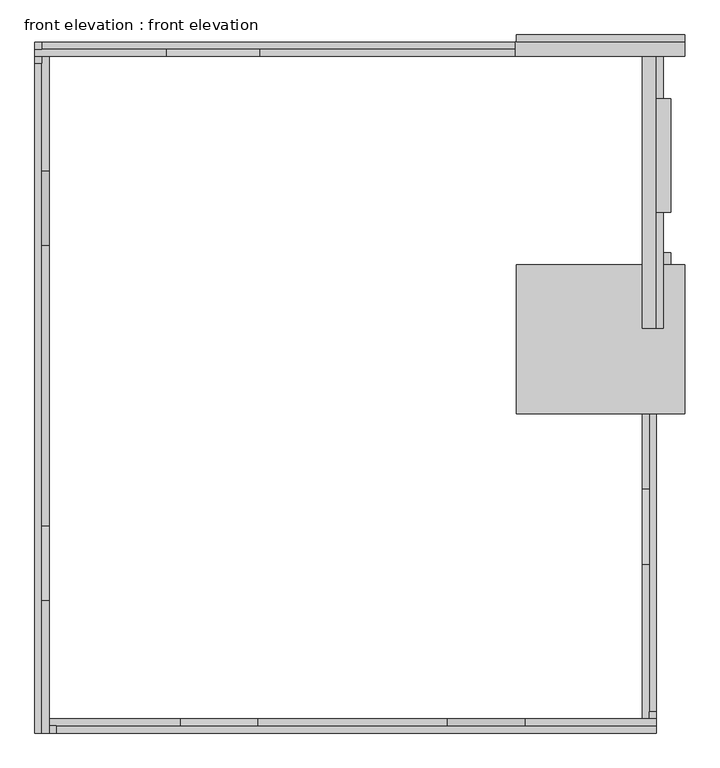
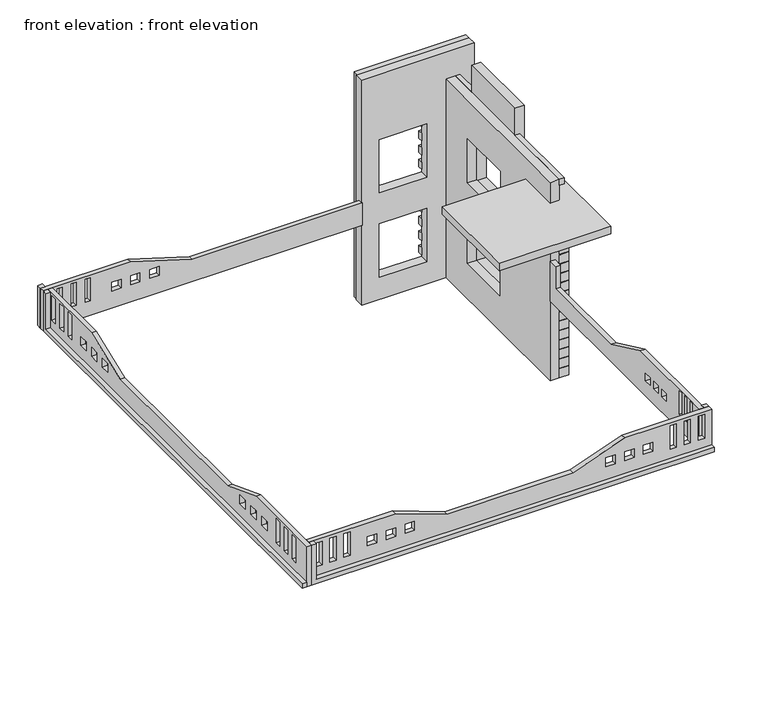
"""IFC4 building model written with IfcOpenShell, lengths in millimetres: proxy geometry, front elevation : front elevation."""

from ifc_helpers import new_model, si_unit, frame, origin, origin_with_axes, place, context, project, spatial, polyline, outline, extrude, source, transform, mapped, element, save


def front_elevation_front_elevation_9f25110b(model_context):
    return source(origin(), model_context, "Body", "SweptSolid", [
        extrude(outline(polyline([(2743.2, -12805.1277598), (2743.2, -2441.9277598), (2895.6, -2441.9277598), (2895.6, -12652.7277598), (4114.8, -12652.7277598), (4114.8, -12805.1277598), (2743.2, -12805.1277598)])), frame((0.0, 12133.2342801, 0.0), z_axis=(0.0, 1.0, 0.0), x_axis=(0.0, 0.0, 1.0)), (0.0, 0.0, 1.0), 152.4),
        extrude(outline(polyline([(4114.8, -12805.1277598), (2743.2, -12805.1277598), (2743.2, -2441.9277598), (3505.2, -2441.9277598), (3505.2, -7971.0820996), (4114.8, -9964.9938558), (4114.8, -12805.1277598)]), holes=[polyline([(4030.2654166, -12342.301337), (4030.2654166, -12189.901337), (3242.8654166, -12189.901337), (3242.8654166, -12342.301337), (4030.2654166, -12342.301337)]), polyline([(4030.2654166, -11885.101337), (4030.2654166, -11732.701337), (3242.8654166, -11732.701337), (3242.8654166, -11885.101337), (4030.2654166, -11885.101337)]), polyline([(4030.2654166, -11427.901337), (4030.2654166, -11275.501337), (3242.8654166, -11275.501337), (3242.8654166, -11427.901337), (4030.2654166, -11427.901337)]), polyline([(3632.4929332, -10574.5938558), (3632.4929332, -10269.7938558), (3327.6929332, -10269.7938558), (3327.6929332, -10574.5938558), (3632.4929332, -10574.5938558)]), polyline([(3632.4929332, -9964.9938558), (3632.4929332, -9660.1938558), (3327.6929332, -9660.1938558), (3327.6929332, -9964.9938558), (3632.4929332, -9964.9938558)]), polyline([(3632.4929332, -9338.0277598), (3632.4929332, -9033.2277598), (3327.6929332, -9033.2277598), (3327.6929332, -9338.0277598), (3632.4929332, -9338.0277598)])]), frame((0.0, 11980.8342801, 0.0), z_axis=(0.0, 1.0, 0.0), x_axis=(0.0, 0.0, 1.0)), (0.0, 0.0, 1.0), 152.4),
        extrude(outline(polyline([(-2573.3657199, 2895.6), (11828.4342801, 2895.6), (11828.4342801, 4114.8), (11980.8342801, 4114.8), (11980.8342801, 2743.2), (-2573.3657199, 2743.2), (-2573.3657199, 2895.6)])), frame((-12805.1277598, 0.0, 0.0), z_axis=(1.0, 0.0, 0.0), x_axis=(0.0, 1.0, 0.0)), (0.0, 0.0, 1.0), 152.4),
        extrude(outline(polyline([(9519.971833, 4114.8), (11980.8342801, 4114.8), (11980.8342801, 2743.2), (-2573.3657199, 2743.2), (-2573.3657199, 4114.8), (268.4967273, 4114.8), (1879.1217625, 3505.2), (7909.3467978, 3505.2), (9519.971833, 4114.8)]), holes=[polyline([(11549.0342801, 4034.6754995), (11549.0342801, 3200.4), (11752.2342801, 3200.4), (11752.2342801, 4034.6754995), (11549.0342801, 4034.6754995)]), polyline([(11091.8342801, 4034.6754995), (11091.8342801, 3200.4), (11295.0342801, 3200.4), (11295.0342801, 4034.6754995), (11091.8342801, 4034.6754995)]), polyline([(10634.6342801, 4034.6754995), (10634.6342801, 3200.4), (10837.8342801, 3200.4), (10837.8342801, 4034.6754995), (10634.6342801, 4034.6754995)]), polyline([(9824.771833, 3617.7710854), (9824.771833, 3312.9710854), (10129.571833, 3312.9710854), (10129.571833, 3617.7710854), (9824.771833, 3617.7710854)]), polyline([(9215.171833, 3617.7710854), (9215.171833, 3312.9710854), (9519.971833, 3312.9710854), (9519.971833, 3617.7710854), (9215.171833, 3617.7710854)]), polyline([(8605.571833, 3617.7710854), (8605.571833, 3312.9710854), (8910.371833, 3312.9710854), (8910.371833, 3617.7710854), (8605.571833, 3617.7710854)]), polyline([(-1760.5657199, 4034.6754995), (-1963.7657199, 4034.6754995), (-1963.7657199, 3200.4), (-1760.5657199, 3200.4), (-1760.5657199, 4034.6754995)]), polyline([(-1303.3657199, 4034.6754995), (-1506.5657199, 4034.6754995), (-1506.5657199, 3200.4), (-1303.3657199, 3200.4), (-1303.3657199, 4034.6754995)]), polyline([(-846.1657199, 4034.6754995), (-1049.3657199, 4034.6754995), (-1049.3657199, 3200.4), (-846.1657199, 3200.4), (-846.1657199, 4034.6754995)]), polyline([(-36.3032727, 3617.7710854), (-341.1032727, 3617.7710854), (-341.1032727, 3312.9710854), (-36.3032727, 3312.9710854), (-36.3032727, 3617.7710854)]), polyline([(573.2967273, 3617.7710854), (268.4967273, 3617.7710854), (268.4967273, 3312.9710854), (573.2967273, 3312.9710854), (573.2967273, 3617.7710854)]), polyline([(1182.8967273, 3617.7710854), (878.0967273, 3617.7710854), (878.0967273, 3312.9710854), (1182.8967273, 3312.9710854), (1182.8967273, 3617.7710854)])]), frame((-12652.7277598, 0.0, 0.0), z_axis=(1.0, 0.0, 0.0), x_axis=(0.0, 1.0, 0.0)), (0.0, 0.0, 1.0), 152.4),
        extrude(outline(polyline([(2895.6, 567.9722402), (2895.6, -12347.9277598), (4114.8, -12347.9277598), (4114.8, -12500.3277598), (2743.2, -12500.3277598), (2743.2, 567.9722402), (2895.6, 567.9722402)])), frame((0.0, -2573.3657199, 0.0), z_axis=(0.0, 1.0, 0.0), x_axis=(0.0, 0.0, 1.0)), (0.0, 0.0, 1.0), 152.4),
        extrude(outline(polyline([(4114.8, -9680.4637674), (4114.8, -12500.3277598), (2743.2, -12500.3277598), (2743.2, 567.9722402), (4114.8, 567.9722402), (4114.8, -2251.8917521), (3505.2, -3926.753987), (3505.2, -8005.6015325), (4114.8, -9680.4637674)]), holes=[polyline([(4009.3182057, -12068.5277598), (3200.4, -12068.5277598), (3200.4, -12271.7277598), (4009.3182057, -12271.7277598), (4009.3182057, -12068.5277598)]), polyline([(4009.3182057, -11611.3277598), (3200.4, -11611.3277598), (3200.4, -11814.5277598), (4009.3182057, -11814.5277598), (4009.3182057, -11611.3277598)]), polyline([(4009.3182057, -11154.1277598), (3200.4, -11154.1277598), (3200.4, -11357.3277598), (4009.3182057, -11357.3277598), (4009.3182057, -11154.1277598)]), polyline([(3637.4565129, -10290.0637674), (3332.6565129, -10290.0637674), (3332.6565129, -10594.8637674), (3637.4565129, -10594.8637674), (3637.4565129, -10290.0637674)]), polyline([(3637.4565129, -9680.4637674), (3332.6565129, -9680.4637674), (3332.6565129, -9985.2637674), (3637.4565129, -9985.2637674), (3637.4565129, -9680.4637674)]), polyline([(3637.4565129, -9070.8637674), (3332.6565129, -9070.8637674), (3332.6565129, -9375.6637674), (3637.4565129, -9375.6637674), (3637.4565129, -9070.8637674)]), polyline([(4009.3182057, 136.1722402), (4009.3182057, 339.3722402), (3200.4, 339.3722402), (3200.4, 136.1722402), (4009.3182057, 136.1722402)]), polyline([(4009.3182057, -321.0277598), (4009.3182057, -117.8277598), (3200.4, -117.8277598), (3200.4, -321.0277598), (4009.3182057, -321.0277598)]), polyline([(4009.3182057, -778.2277598), (4009.3182057, -575.0277598), (3200.4, -575.0277598), (3200.4, -778.2277598), (4009.3182057, -778.2277598)]), polyline([(3637.4565129, -1642.2917521), (3637.4565129, -1337.4917521), (3332.6565129, -1337.4917521), (3332.6565129, -1642.2917521), (3637.4565129, -1642.2917521)]), polyline([(3637.4565129, -2251.8917521), (3637.4565129, -1947.0917521), (3332.6565129, -1947.0917521), (3332.6565129, -2251.8917521), (3637.4565129, -2251.8917521)]), polyline([(3637.4565129, -2861.4917521), (3637.4565129, -2556.6917521), (3332.6565129, -2556.6917521), (3332.6565129, -2861.4917521), (3637.4565129, -2861.4917521)])]), frame((0.0, -2420.9657199, 0.0), z_axis=(0.0, 1.0, 0.0), x_axis=(0.0, 0.0, 1.0)), (0.0, 0.0, 1.0), 152.4),
        extrude(outline(polyline([(6113.4342801, 2743.2), (-2268.5657199, 2743.2), (-2268.5657199, 4114.8), (-2116.1657199, 4114.8), (-2116.1657199, 2892.3381974), (6113.4342801, 2892.3381974), (6113.4342801, 2743.2)])), frame((415.5722402, 0.0, 0.0), z_axis=(1.0, 0.0, 0.0), x_axis=(0.0, 1.0, 0.0)), (0.0, 0.0, 1.0), 152.4),
        extrude(outline(polyline([(1046.1342801, 4114.8), (2680.2485536, 3352.8), (5808.6342801, 3352.8), (5808.6342801, 4114.8), (6113.4342801, 4114.8), (6113.4342801, 2743.2), (-2268.5657199, 2743.2), (-2268.5657199, 4114.8), (1046.1342801, 4114.8)]), holes=[polyline([(-1737.5236291, 4073.1188318), (-1864.5236291, 4073.1188318), (-1864.5236291, 3260.3188318), (-1737.5236291, 3260.3188318), (-1737.5236291, 4073.1188318)]), polyline([(-1432.7236291, 4073.1188318), (-1559.7236291, 4073.1188318), (-1559.7236291, 3260.3188318), (-1432.7236291, 3260.3188318), (-1432.7236291, 4073.1188318)]), polyline([(-1138.2657199, 4073.1188318), (-1265.2657199, 4073.1188318), (-1265.2657199, 3260.3188318), (-1138.2657199, 3260.3188318), (-1138.2657199, 4073.1188318)]), polyline([(-149.6119019, 3260.3188318), (-149.6119019, 3514.3188318), (-403.6119019, 3514.3188318), (-403.6119019, 3260.3188318), (-149.6119019, 3260.3188318)]), polyline([(307.5880981, 3260.3188318), (307.5880981, 3514.3188318), (53.5880981, 3514.3188318), (53.5880981, 3260.3188318), (307.5880981, 3260.3188318)]), polyline([(764.7880981, 3260.3188318), (764.7880981, 3514.3188318), (510.7880981, 3514.3188318), (510.7880981, 3260.3188318), (764.7880981, 3260.3188318)])]), frame((263.1722402, 0.0, 0.0), z_axis=(1.0, 0.0, 0.0), x_axis=(0.0, 1.0, 0.0)), (0.0, 0.0, 1.0), 152.4),
        extrude(outline(polyline([(-349.3883629, 12438.0342801), (872.7722402, 12438.0342801), (872.7722402, 12285.6342801), (-349.3883629, 12285.6342801), (-349.3883629, 12438.0342801)])), frame((0.0, 0.0, 794.6571429), z_axis=(0.0, 0.0, 1.0), x_axis=(1.0, 0.0, 0.0)), (0.0, 0.0, 1.0), 254.0),
        extrude(outline(polyline([(-349.3883629, 12438.0342801), (872.7722402, 12438.0342801), (872.7722402, 12285.6342801), (-349.3883629, 12285.6342801), (-349.3883629, 12438.0342801)])), frame((0.0, 0.0, 1284.5142857), z_axis=(0.0, 0.0, 1.0), x_axis=(1.0, 0.0, 0.0)), (0.0, 0.0, 1.0), 254.0),
        extrude(outline(polyline([(-349.3883629, 12438.0342801), (872.7722402, 12438.0342801), (872.7722402, 12285.6342801), (-349.3883629, 12285.6342801), (-349.3883629, 12438.0342801)])), frame((0.0, 0.0, 1774.3714286), z_axis=(0.0, 0.0, 1.0), x_axis=(1.0, 0.0, 0.0)), (0.0, 0.0, 1.0), 254.0),
        extrude(outline(polyline([(-349.3883629, 12438.0342801), (872.7722402, 12438.0342801), (872.7722402, 12285.6342801), (-349.3883629, 12285.6342801), (-349.3883629, 12438.0342801)])), frame((0.0, 0.0, 2264.2285714), z_axis=(0.0, 0.0, 1.0), x_axis=(1.0, 0.0, 0.0)), (0.0, 0.0, 1.0), 254.0),
        extrude(outline(polyline([(-2137.1277598, 12438.0342801), (872.7722402, 12438.0342801), (872.7722402, 12285.6342801), (-2137.1277598, 12285.6342801), (-2137.1277598, 12438.0342801)])), frame((0.0, 0.0, 2754.0857143), z_axis=(0.0, 0.0, 1.0), x_axis=(1.0, 0.0, 0.0)), (0.0, 0.0, 1.0), 254.0),
        extrude(outline(polyline([(-2137.1277598, 12438.0342801), (872.7722402, 12438.0342801), (872.7722402, 12285.6342801), (-2137.1277598, 12285.6342801), (-2137.1277598, 12438.0342801)])), frame((0.0, 0.0, 3243.9428571), z_axis=(0.0, 0.0, 1.0), x_axis=(1.0, 0.0, 0.0)), (0.0, 0.0, 1.0), 254.0),
        extrude(outline(polyline([(-349.3883629, 12438.0342801), (872.7722402, 12438.0342801), (872.7722402, 12285.6342801), (-349.3883629, 12285.6342801), (-349.3883629, 12438.0342801)])), frame((0.0, 0.0, 3733.8), z_axis=(0.0, 0.0, 1.0), x_axis=(1.0, 0.0, 0.0)), (0.0, 0.0, 1.0), 254.0),
        extrude(outline(polyline([(-349.3883629, 12438.0342801), (872.7722402, 12438.0342801), (872.7722402, 12285.6342801), (-349.3883629, 12285.6342801), (-349.3883629, 12438.0342801)])), frame((0.0, 0.0, 4223.6571429), z_axis=(0.0, 0.0, 1.0), x_axis=(1.0, 0.0, 0.0)), (0.0, 0.0, 1.0), 254.0),
        extrude(outline(polyline([(-349.3883629, 12438.0342801), (872.7722402, 12438.0342801), (872.7722402, 12285.6342801), (-349.3883629, 12285.6342801), (-349.3883629, 12438.0342801)])), frame((0.0, 0.0, 4713.5142857), z_axis=(0.0, 0.0, 1.0), x_axis=(1.0, 0.0, 0.0)), (0.0, 0.0, 1.0), 254.0),
        extrude(outline(polyline([(-349.3883629, 12438.0342801), (872.7722402, 12438.0342801), (872.7722402, 12285.6342801), (-349.3883629, 12285.6342801), (-349.3883629, 12438.0342801)])), frame((0.0, 0.0, 5203.3714286), z_axis=(0.0, 0.0, 1.0), x_axis=(1.0, 0.0, 0.0)), (0.0, 0.0, 1.0), 254.0),
        extrude(outline(polyline([(-2137.1277598, 12438.0342801), (872.7722402, 12438.0342801), (872.7722402, 12285.6342801), (-2137.1277598, 12285.6342801), (-2137.1277598, 12438.0342801)])), frame((0.0, 0.0, 5693.2285714), z_axis=(0.0, 0.0, 1.0), x_axis=(1.0, 0.0, 0.0)), (0.0, 0.0, 1.0), 254.0),
        extrude(outline(polyline([(-2137.1277598, 12438.0342801), (872.7722402, 12438.0342801), (872.7722402, 12285.6342801), (-2137.1277598, 12285.6342801), (-2137.1277598, 12438.0342801)])), frame((0.0, 0.0, 6183.0857143), z_axis=(0.0, 0.0, 1.0), x_axis=(1.0, 0.0, 0.0)), (0.0, 0.0, 1.0), 254.0),
        extrude(outline(polyline([(-2137.1277598, 12438.0342801), (872.7722402, 12438.0342801), (872.7722402, 12285.6342801), (-2137.1277598, 12285.6342801), (-2137.1277598, 12438.0342801)])), frame((0.0, 0.0, 6672.9428571), z_axis=(0.0, 0.0, 1.0), x_axis=(1.0, 0.0, 0.0)), (0.0, 0.0, 1.0), 254.0),
        extrude(outline(polyline([(-2137.1277598, 12438.0342801), (872.7722402, 12438.0342801), (872.7722402, 12285.6342801), (-2137.1277598, 12285.6342801), (-2137.1277598, 12438.0342801)])), frame((0.0, 0.0, 304.8), z_axis=(0.0, 0.0, 1.0), x_axis=(1.0, 0.0, 0.0)), (0.0, 0.0, 1.0), 254.0),
        extrude(outline(polyline([(-2137.1277598, 12438.0342801), (872.7722402, 12438.0342801), (872.7722402, 12285.6342801), (-2137.1277598, 12285.6342801), (-2137.1277598, 12438.0342801)])), frame((0.0, 0.0, 7162.8), z_axis=(0.0, 0.0, 1.0), x_axis=(1.0, 0.0, 0.0)), (0.0, 0.0, 1.0), 254.0),
        extrude(outline(polyline([(7721.6, -2441.9277598), (0.0, -2441.9277598), (0.0, 1177.5722402), (7721.6, 1177.5722402), (7721.6, -2441.9277598)]), holes=[polyline([(7416.8, -2137.1277598), (7416.8, 872.7722402), (304.8, 872.7722402), (304.8, -2137.1277598), (7416.8, -2137.1277598)])]), frame((0.0, 12285.6342801, 0.0), z_axis=(0.0, 1.0, 0.0), x_axis=(0.0, 0.0, 1.0)), (0.0, 0.0, 1.0), 152.4),
        extrude(outline(polyline([(7721.6, -2461.9277598), (0.0, -2461.9277598), (0.0, 1177.5722402), (7721.6, 1177.5722402), (7721.6, -2461.9277598)]), holes=[polyline([(762.0, -349.3883629), (762.0, -1897.2923825), (2590.8, -1897.2923825), (2590.8, -349.3883629), (762.0, -349.3883629)]), polyline([(3657.6, -349.3883629), (3657.6, -1897.2923825), (5486.4, -1897.2923825), (5486.4, -349.3883629), (3657.6, -349.3883629)])]), frame((0.0, 11980.8342801, 0.0), z_axis=(0.0, 1.0, 0.0), x_axis=(0.0, 0.0, 1.0)), (0.0, 0.0, 1.0), 304.8),
        extrude(outline(polyline([(720.3722402, 8628.0342801), (720.3722402, 6126.1342801), (567.9722402, 6126.1342801), (567.9722402, 8628.0342801), (720.3722402, 8628.0342801)])), frame((0.0, 0.0, 6604.0), z_axis=(0.0, 0.0, 1.0), x_axis=(1.0, 0.0, 0.0)), (0.0, 0.0, 1.0), 203.2),
        extrude(outline(polyline([(720.3722402, 11980.8342801), (720.3722402, 11066.4342801), (567.9722402, 11066.4342801), (567.9722402, 11980.8342801), (720.3722402, 11980.8342801)])), frame((0.0, 0.0, 6592.15659), z_axis=(0.0, 0.0, 1.0), x_axis=(1.0, 0.0, 0.0)), (0.0, 0.0, 1.0), 215.04341),
        extrude(outline(polyline([(872.7722402, 7495.8277491), (872.7722402, 6126.1342801), (567.9722402, 6126.1342801), (567.9722402, 7495.8277491), (872.7722402, 7495.8277491)])), frame((0.0, 0.0, 325.7176471), z_axis=(0.0, 0.0, 1.0), x_axis=(1.0, 0.0, 0.0)), (0.0, 0.0, 1.0), 304.8),
        extrude(outline(polyline([(872.7722402, 7495.8277491), (872.7722402, 6126.1342801), (567.9722402, 6126.1342801), (567.9722402, 7495.8277491), (872.7722402, 7495.8277491)])), frame((0.0, 0.0, 651.4352941), z_axis=(0.0, 0.0, 1.0), x_axis=(1.0, 0.0, 0.0)), (0.0, 0.0, 1.0), 304.8),
        extrude(outline(polyline([(872.7722402, 7495.8277491), (872.7722402, 6126.1342801), (567.9722402, 6126.1342801), (567.9722402, 7495.8277491), (872.7722402, 7495.8277491)])), frame((0.0, 0.0, 977.1529412), z_axis=(0.0, 0.0, 1.0), x_axis=(1.0, 0.0, 0.0)), (0.0, 0.0, 1.0), 304.8),
        extrude(outline(polyline([(872.7722402, 7495.8277491), (872.7722402, 6126.1342801), (567.9722402, 6126.1342801), (567.9722402, 7495.8277491), (872.7722402, 7495.8277491)])), frame((0.0, 0.0, 1302.8705882), z_axis=(0.0, 0.0, 1.0), x_axis=(1.0, 0.0, 0.0)), (0.0, 0.0, 1.0), 304.8),
        extrude(outline(polyline([(872.7722402, 7495.8277491), (872.7722402, 6126.1342801), (567.9722402, 6126.1342801), (567.9722402, 7495.8277491), (872.7722402, 7495.8277491)])), frame((0.0, 0.0, 1628.5882353), z_axis=(0.0, 0.0, 1.0), x_axis=(1.0, 0.0, 0.0)), (0.0, 0.0, 1.0), 304.8),
        extrude(outline(polyline([(872.7722402, 7495.8277491), (872.7722402, 6126.1342801), (567.9722402, 6126.1342801), (567.9722402, 7495.8277491), (872.7722402, 7495.8277491)])), frame((0.0, 0.0, 1954.3058824), z_axis=(0.0, 0.0, 1.0), x_axis=(1.0, 0.0, 0.0)), (0.0, 0.0, 1.0), 304.8),
        extrude(outline(polyline([(872.7722402, 7495.8277491), (872.7722402, 6126.1342801), (567.9722402, 6126.1342801), (567.9722402, 7495.8277491), (872.7722402, 7495.8277491)])), frame((0.0, 0.0, 2280.0235294), z_axis=(0.0, 0.0, 1.0), x_axis=(1.0, 0.0, 0.0)), (0.0, 0.0, 1.0), 304.8),
        extrude(outline(polyline([(872.7722402, 7495.8277491), (872.7722402, 6126.1342801), (567.9722402, 6126.1342801), (567.9722402, 7495.8277491), (872.7722402, 7495.8277491)])), frame((0.0, 0.0, 2605.7411765), z_axis=(0.0, 0.0, 1.0), x_axis=(1.0, 0.0, 0.0)), (0.0, 0.0, 1.0), 304.8),
        extrude(outline(polyline([(872.7722402, 7495.8277491), (872.7722402, 6126.1342801), (567.9722402, 6126.1342801), (567.9722402, 7495.8277491), (872.7722402, 7495.8277491)])), frame((0.0, 0.0, 2931.4588235), z_axis=(0.0, 0.0, 1.0), x_axis=(1.0, 0.0, 0.0)), (0.0, 0.0, 1.0), 304.8),
        extrude(outline(polyline([(872.7722402, 7495.8277491), (872.7722402, 6126.1342801), (567.9722402, 6126.1342801), (567.9722402, 7495.8277491), (872.7722402, 7495.8277491)])), frame((0.0, 0.0, 3257.1764706), z_axis=(0.0, 0.0, 1.0), x_axis=(1.0, 0.0, 0.0)), (0.0, 0.0, 1.0), 304.8),
        extrude(outline(polyline([(872.7722402, 7495.8277491), (872.7722402, 6126.1342801), (567.9722402, 6126.1342801), (567.9722402, 7495.8277491), (872.7722402, 7495.8277491)])), frame((0.0, 0.0, 3582.8941176), z_axis=(0.0, 0.0, 1.0), x_axis=(1.0, 0.0, 0.0)), (0.0, 0.0, 1.0), 304.8),
        extrude(outline(polyline([(872.7722402, 7495.8277491), (872.7722402, 6126.1342801), (567.9722402, 6126.1342801), (567.9722402, 7495.8277491), (872.7722402, 7495.8277491)])), frame((0.0, 0.0, 3908.6117647), z_axis=(0.0, 0.0, 1.0), x_axis=(1.0, 0.0, 0.0)), (0.0, 0.0, 1.0), 304.8),
        extrude(outline(polyline([(872.7722402, 7495.8277491), (872.7722402, 6126.1342801), (567.9722402, 6126.1342801), (567.9722402, 7495.8277491), (872.7722402, 7495.8277491)])), frame((0.0, 0.0, 4234.3294118), z_axis=(0.0, 0.0, 1.0), x_axis=(1.0, 0.0, 0.0)), (0.0, 0.0, 1.0), 304.8),
        extrude(outline(polyline([(872.7722402, 7495.8277491), (872.7722402, 6126.1342801), (567.9722402, 6126.1342801), (567.9722402, 7495.8277491), (872.7722402, 7495.8277491)])), frame((0.0, 0.0, 4560.0470588), z_axis=(0.0, 0.0, 1.0), x_axis=(1.0, 0.0, 0.0)), (0.0, 0.0, 1.0), 304.8),
        extrude(outline(polyline([(872.7722402, 7495.8277491), (872.7722402, 6126.1342801), (567.9722402, 6126.1342801), (567.9722402, 7495.8277491), (872.7722402, 7495.8277491)])), frame((0.0, 0.0, 4885.7647059), z_axis=(0.0, 0.0, 1.0), x_axis=(1.0, 0.0, 0.0)), (0.0, 0.0, 1.0), 304.8),
        extrude(outline(polyline([(872.7722402, 7495.8277491), (872.7722402, 6126.1342801), (567.9722402, 6126.1342801), (567.9722402, 7495.8277491), (872.7722402, 7495.8277491)])), frame((0.0, 0.0, 5211.4823529), z_axis=(0.0, 0.0, 1.0), x_axis=(1.0, 0.0, 0.0)), (0.0, 0.0, 1.0), 304.8),
        extrude(outline(polyline([(872.7722402, 7495.8277491), (872.7722402, 6126.1342801), (567.9722402, 6126.1342801), (567.9722402, 7495.8277491), (872.7722402, 7495.8277491)])), origin_with_axes(), (0.0, 0.0, 1.0), 304.8),
        extrude(outline(polyline([(872.7722402, 7495.8277491), (872.7722402, 6126.1342801), (567.9722402, 6126.1342801), (567.9722402, 7495.8277491), (872.7722402, 7495.8277491)])), frame((0.0, 0.0, 5537.2), z_axis=(0.0, 0.0, 1.0), x_axis=(1.0, 0.0, 0.0)), (0.0, 0.0, 1.0), 304.8),
        extrude(outline(polyline([(1177.5722402, 7495.8277491), (1177.5722402, 4297.3342801), (-2441.9277598, 4297.3342801), (-2441.9277598, 7495.8277491), (1177.5722402, 7495.8277491)])), frame((0.0, 0.0, 5842.0), z_axis=(0.0, 0.0, 1.0), x_axis=(1.0, 0.0, 0.0)), (0.0, 0.0, 1.0), 254.0),
        extrude(outline(polyline([(872.7722402, 10761.6342801), (872.7722402, 8932.8342801), (567.9722402, 8932.8342801), (567.9722402, 10761.6342801), (872.7722402, 10761.6342801)])), frame((0.0, 0.0, 3021.0087041), z_axis=(0.0, 0.0, 1.0), x_axis=(1.0, 0.0, 0.0)), (0.0, 0.0, 1.0), 101.6),
        extrude(outline(polyline([(872.7722402, 10761.6342801), (872.7722402, 8932.8342801), (567.9722402, 8932.8342801), (567.9722402, 10761.6342801), (872.7722402, 10761.6342801)])), frame((0.0, 0.0, 3298.8174081), z_axis=(0.0, 0.0, 1.0), x_axis=(1.0, 0.0, 0.0)), (0.0, 0.0, 1.0), 101.6),
        extrude(outline(polyline([(872.7722402, 10761.6342801), (872.7722402, 8932.8342801), (567.9722402, 8932.8342801), (567.9722402, 10761.6342801), (872.7722402, 10761.6342801)])), frame((0.0, 0.0, 3576.6261122), z_axis=(0.0, 0.0, 1.0), x_axis=(1.0, 0.0, 0.0)), (0.0, 0.0, 1.0), 101.6),
        extrude(outline(polyline([(872.7722402, 10761.6342801), (872.7722402, 8932.8342801), (567.9722402, 8932.8342801), (567.9722402, 10761.6342801), (872.7722402, 10761.6342801)])), frame((0.0, 0.0, 2743.2), z_axis=(0.0, 0.0, 1.0), x_axis=(1.0, 0.0, 0.0)), (0.0, 0.0, 1.0), 101.6),
        extrude(outline(polyline([(872.7722402, 10761.6342801), (872.7722402, 8932.8342801), (567.9722402, 8932.8342801), (567.9722402, 10761.6342801), (872.7722402, 10761.6342801)])), frame((0.0, 0.0, 3854.4348163), z_axis=(0.0, 0.0, 1.0), x_axis=(1.0, 0.0, 0.0)), (0.0, 0.0, 1.0), 101.6),
        extrude(outline(polyline([(11066.4342801, 7721.6), (11066.4342801, 914.4), (8628.0342801, 914.4), (8628.0342801, 7721.6), (11066.4342801, 7721.6)]), holes=[polyline([(10761.6342801, 5486.4), (8932.8342801, 5486.4), (8932.8342801, 1219.2), (10761.6342801, 1219.2), (10761.6342801, 5486.4)])]), frame((567.9722402, 0.0, 0.0), z_axis=(1.0, 0.0, 0.0), x_axis=(0.0, 1.0, 0.0)), (0.0, 0.0, 1.0), 304.8),
        extrude(outline(polyline([(7749.8277491, 6096.0), (7749.8277491, -152.4), (7495.8277491, -152.4), (7495.8277491, 5842.0), (6126.1342801, 5842.0), (6126.1342801, 6096.0), (7749.8277491, 6096.0)])), frame((567.9722402, 0.0, 0.0), z_axis=(1.0, 0.0, 0.0), x_axis=(0.0, 1.0, 0.0)), (0.0, 0.0, 1.0), 304.8),
        extrude(outline(polyline([(11980.8342801, 6807.2), (11980.8342801, 0.0), (6126.1342801, 0.0), (6126.1342801, 6807.2), (11980.8342801, 6807.2)]), holes=[polyline([(10766.7142801, 5500.7979445), (8927.7542801, 5500.7979445), (8927.7542801, 3976.7979445), (10766.7142801, 3976.7979445), (10766.7142801, 5500.7979445)]), polyline([(8943.6292801, 1217.3131867), (10766.7142801, 1217.3131867), (10766.7142801, 2741.3131867), (8943.6292801, 2741.3131867), (8943.6292801, 1217.3131867)])]), frame((263.1722402, 0.0, 0.0), z_axis=(1.0, 0.0, 0.0), x_axis=(0.0, 1.0, 0.0)), (0.0, 0.0, 1.0), 304.8),
    ])


if __name__ == "__main__":
    model = new_model("IFC4")
    model_context = context("Model", 3, world=origin())
    ifc_project = project(units=[si_unit("LENGTHUNIT", "METRE", prefix="MILLI")], contexts=[model_context])
    site = spatial("IfcSite", under=ifc_project)
    building = spatial("IfcBuilding", under=site)
    placement = place(None, origin())
    front_elevation_front_elevation_shape = front_elevation_front_elevation_9f25110b(model_context)
    element("IfcBuildingElementProxy", 1, Name="front elevation : front elevation", ObjectType="front elevation : front elevation", at=placement, inside=building, context=model_context, shape_type="MappedRepresentation", body=[
        mapped(front_elevation_front_elevation_shape, transform((0.0, 0.0, 0.0), x_axis=(1.0, 0.0, 0.0), y_axis=(0.0, 1.0, 0.0), z_axis=(0.0, 0.0, 1.0))),
    ])
    save(model, "model.ifc")
